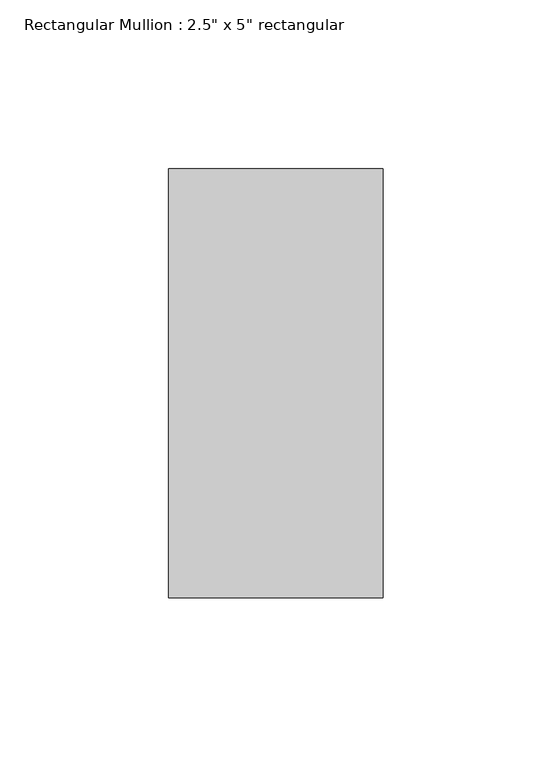
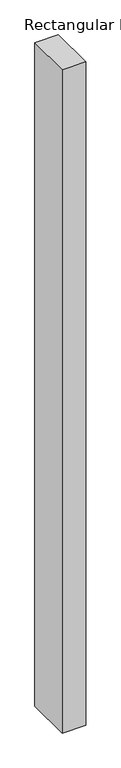
"""IFC4 building model written with IfcOpenShell, lengths in millimetres: member geometry."""

from ifc_helpers import new_model, si_unit, frame, origin, place, context, project, spatial, polyline, outline, extrude, source, transform, mapped, element, save


def member_7b893d20(model_context):
    return source(origin(), model_context, "Body", "SweptSolid", [
        extrude(outline(polyline([(0.0, 63.5), (0.0, -63.5), (-63.5, -63.5), (-63.5, 63.5), (0.0, 63.5)])), frame((0.0, 0.0, -1892.3110628), z_axis=(0.0, 0.0, 1.0), x_axis=(1.0, 0.0, 0.0)), (0.0, 0.0, 1.0), 1892.3110628),
    ])


if __name__ == "__main__":
    model = new_model("IFC4")
    model_context = context("Model", 3, world=origin())
    ifc_project = project(units=[si_unit("LENGTHUNIT", "METRE", prefix="MILLI")], contexts=[model_context])
    site = spatial("IfcSite", under=ifc_project)
    building = spatial("IfcBuilding", under=site)
    placement = place(None, origin())
    member_shape = member_7b893d20(model_context)
    element("IfcMember", 1, ObjectType="Rectangular Mullion : 2.5\" x 5\" rectangular", at=placement, inside=building, context=model_context, shape_type="MappedRepresentation", body=[
        mapped(member_shape, transform((0.0, 0.0, 0.0), x_axis=(1.0, 0.0, 0.0), y_axis=(0.0, 1.0, 0.0), z_axis=(0.0, 0.0, 1.0))),
    ])
    save(model, "model.ifc")

# Revit data of these elements
# Type "Rectangular Mullion : 2.5\" x 5\" rectangular"
#   built-in parameter 1007304 = 0.416667 (stored number, unit not read)
#   built-in parameter 1007301 = 0.104167 (stored number, unit not read)
#   built-in parameter 1007300 = 0.104167 (stored number, unit not read)
# Element 1 (IfcMember, "Rectangular Mullion : 2.5\" x 5\" rectangular")
#   Materials on its faces: "Iron, Ductile"
# Materials
#   "Iron, Ductile": class "Metal", colour RGB 0 0 0, transparency 0, Description = "Ductile cast iron", Cost = 0
